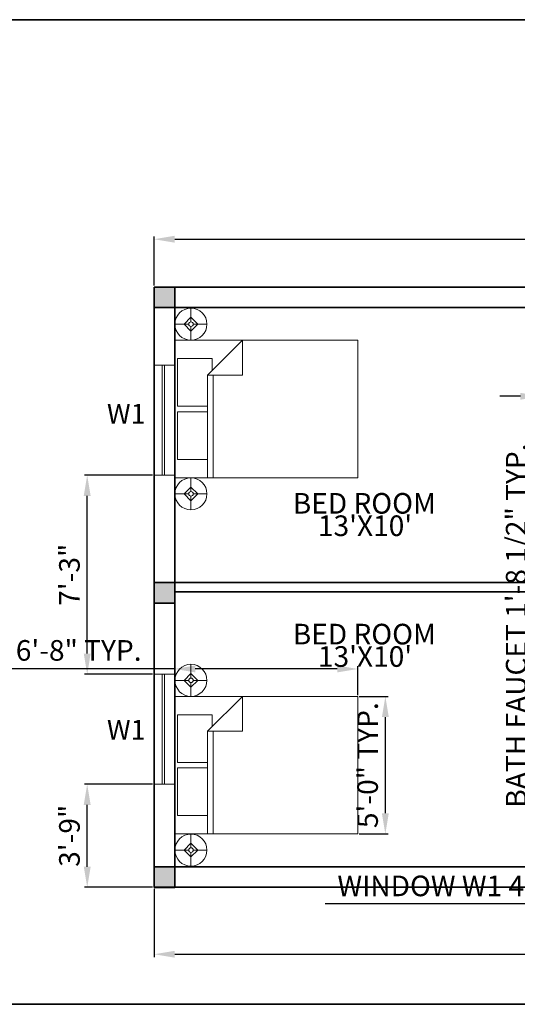
# Model space of a CAD drawing. Units: inches. Extents: x -281 to 2337, y 1647 to 2113.
# Tile 4 of 6: x 1688 to 1906, y 1674 to 2103. Entities that reach past the tile are written whole.
import ezdxf

# ---------------------------------------------------------------- set-up
doc = ezdxf.new("R2010")
doc.units = ezdxf.units.IN
for name, color, linetype, lineweight in [('A-ANNO-DIMS', 242, 'Continuous', 18), ('A-ANNO-IDEN', 11, 'Continuous', 18), ('A-ANNO-TTLB', 7, 'Continuous', 35), ('A-AREA-IDEN', 7, 'Continuous', 18), ('A-COLS', 1, 'Continuous', 35), ('A-FURN', 8, 'Continuous', 18), ('A-GLAZ', 3, 'Continuous', 18), ('A-WALL', 7, 'Continuous', 35)]:
    doc.layers.add(name, color=color, linetype=linetype, lineweight=lineweight)
doc.styles.get("Standard").update_dxf_attribs({"font": 'arial.ttf'})
doc.dimstyles.new('ISO-25', dxfattribs={"dimtxt": 9, "dimasz": 9, "dimexe": 1.25, "dimexo": 0.625, "dimgap": 2, "dimtad": 1, "dimdec": 1, "dimlunit": 4, "dimtxsty": 'Standard', "dimcen": 2.5, "dimadec": 0, "dimazin": 0, "dimtfac": 1, "dimtdec": 1, "dimtmove": 0, "dimatfit": 3, "dimfxl": 1, "dimarcsym": 0})

# ---------------------------------------------------------------- blocks, each defined once
blk = doc.blocks.new('Bed - Queen')
for p, q in [((0, -80.00003), (0, 0)), ((0, 0), (59.99999, 0)), ((59.99999, 0), (59.99999, -80.00003)), ((7.99999, -1.2), (28.79998, -1.2)), ((7.99999, -14.4), (7.99999, -1.2)), ((28.79998, -1.2), (28.79998, -14.4)), ((31.19999, -1.2), (51.99999, -1.2)), ((31.19999, -14.4), (31.19999, -1.2)), ((51.99999, -1.2), (51.99999, -16.4)), ((0, -14.4), (44.8, -14.4)), ((44.8, -16.8), (0, -16.8)), ((59.99999, -29.6), (44.8, -14.4)), ((44.8, -14.4), (44.8, -29.6)), ((51.99999, -16.4), (46.79936, -16.4)), ((44.8, -29.6), (59.99999, -29.6)), ((59.99999, -80.00003), (0, -80.00003))]:
    blk.add_line(p, q)
blk = doc.blocks.new('Lamp - Table')
for p, q in [((0, 7), (0, 1)), ((-1, 0), (-7, 0)), ((0, 3), (-3, 0)), ((-3, 0), (0, -3)), ((3, 0), (0, 3)), ((0, -3), (3, 0)), ((1, 0), (7, 0)), ((0, -1), (0, -7))]:
    blk.add_line(p, q)
for radius in [7, 1]:
    blk.add_circle((0, 0), radius)
blk = doc.blocks.new('*D10')
at = {"layer": 'A-ANNO-DIMS', "color": 0, "lineweight": -2, "transparency": 16777216}
for p, q in [((1746.88, 1987.41), (1746.88, 2008.91)), ((1755.88, 2007.66), (2231.88, 2007.66)), ((2240.88, 1987.41), (2240.88, 2008.91))]:
    blk.add_line(p, q, dxfattribs=at)
at = {"layer": 'A-ANNO-DIMS', "color": 0, "transparency": 16777216}
for points in [[(1755.88, 2009.16), (1755.88, 2006.16), (1746.88, 2007.66)], [(2231.88, 2009.16), (2231.88, 2006.16), (2240.88, 2007.66)]]:
    blk.add_solid(points, dxfattribs=at)
at = {"layer": 'Defpoints', "color": 0, "transparency": 16777216}
for p in [(2240.88, 2007.66), (1746.88, 1986.79), (2240.88, 1986.79)]:
    blk.add_point(p, dxfattribs=at)
at = {"layer": 'A-ANNO-DIMS', "color": 0, "transparency": 16777216, "insert": (1993.88, 2014.18), "char_height": 9, "attachment_point": 5}
blk.add_mtext('41\'-2"', dxfattribs=at)
blk = doc.blocks.new('COL-9x9')
h = blk.add_hatch(color=256)
h.dxf.hatch_style = 1
h.paths.add_polyline_path([(9, 9), (0, 9), (0, 0), (9, 0)])
for p, q in [((0, 9), (9, 9)), ((0, 0), (0, 9)), ((9, 9), (9, 0)), ((9, 0), (0, 0))]:
    blk.add_line(p, q)
blk = doc.blocks.new('WIN-W1-48')
for p, q in [((0, 48), (9, 48)), ((3.5, 0), (3.5, 48)), ((4.5, 0), (4.5, 48)), ((0, 0), (9, 0))]:
    blk.add_line(p, q)
blk = doc.blocks.new('*D19')
at = {"layer": 'A-ANNO-DIMS', "color": 0, "lineweight": -2, "transparency": 16777216}
for p, q in [((1970.88, 1724.16), (1970.88, 1716.34)), ((2018.88, 1724.16), (2018.88, 1716.34)), ((1970.88, 1717.59), (1821.64, 1717.59)), ((2009.88, 1717.59), (1979.88, 1717.59))]:
    blk.add_line(p, q, dxfattribs=at)
at = {"layer": 'A-ANNO-DIMS', "color": 0, "transparency": 16777216}
for points in [[(1979.88, 1719.09), (1979.88, 1716.09), (1970.88, 1717.59)], [(2009.88, 1719.09), (2009.88, 1716.09), (2018.88, 1717.59)]]:
    blk.add_solid(points, dxfattribs=at)
at = {"layer": 'Defpoints', "color": 0, "transparency": 16777216}
for p in [(1970.88, 1724.79), (2018.88, 1724.79), (1970.88, 1717.59)]:
    blk.add_point(p, dxfattribs=at)
at = {"layer": 'A-ANNO-DIMS', "color": 0, "transparency": 16777216, "insert": (1891.76, 1724.24), "char_height": 9, "attachment_point": 5}
blk.add_mtext('WINDOW W1 4\'-0" TYP.', dxfattribs=at)
blk = doc.blocks.new('*D25')
at = {"layer": 'A-ANNO-DIMS', "color": 0, "lineweight": -2, "transparency": 16777216}
for p, q in [((1755.88, 1820.1), (1610.49, 1820.1)), ((1755.88, 1808.73), (1755.88, 1821.35)), ((1826.88, 1820.1), (1764.88, 1820.1)), ((1835.88, 1808.73), (1835.88, 1821.35))]:
    blk.add_line(p, q, dxfattribs=at)
at = {"layer": 'A-ANNO-DIMS', "color": 0, "transparency": 16777216}
for points in [[(1764.88, 1821.6), (1764.88, 1818.6), (1755.88, 1820.1)], [(1826.88, 1821.6), (1826.88, 1818.6), (1835.88, 1820.1)]]:
    blk.add_solid(points, dxfattribs=at)
at = {"layer": 'Defpoints', "color": 0, "transparency": 16777216}
for p in [(1755.88, 1820.1), (1755.88, 1808.1), (1835.88, 1808.1)]:
    blk.add_point(p, dxfattribs=at)
at = {"layer": 'A-ANNO-DIMS', "color": 0, "transparency": 16777216, "insert": (1678.68, 1827.03), "char_height": 9, "attachment_point": 5}
blk.add_mtext('QUEEN BED 6\'-8" TYP.', dxfattribs=at)
blk = doc.blocks.new('*D26')
at = {"layer": 'A-ANNO-DIMS', "color": 0, "lineweight": -2, "transparency": 16777216}
for p, q in [((1836.51, 1808.1), (1849.13, 1808.1)), ((1847.88, 1757.1), (1847.88, 1799.1)), ((1836.51, 1748.1), (1849.13, 1748.1))]:
    blk.add_line(p, q, dxfattribs=at)
at = {"layer": 'A-ANNO-DIMS', "color": 0, "transparency": 16777216}
for points in [[(1846.38, 1799.1), (1849.38, 1799.1), (1847.88, 1808.1)], [(1846.38, 1757.1), (1849.38, 1757.1), (1847.88, 1748.1)]]:
    blk.add_solid(points, dxfattribs=at)
at = {"layer": 'Defpoints', "color": 0, "transparency": 16777216}
for p in [(1835.88, 1808.1), (1847.88, 1808.1), (1835.88, 1748.1)]:
    blk.add_point(p, dxfattribs=at)
at = {"layer": 'A-ANNO-DIMS', "color": 0, "transparency": 16777216, "insert": (1841.29, 1778.1), "char_height": 9, "attachment_point": 5, "rotation": 90}
blk.add_mtext('5\'-0" TYP.', dxfattribs=at)
blk = doc.blocks.new('*D39')
at = {"layer": 'A-ANNO-DIMS', "color": 0, "lineweight": -2, "transparency": 16777216}
for p, q in [((1912.84, 1971.43), (1912.84, 1980.43)), ((1915.26, 1962.43), (1911.59, 1962.43)), ((1912.84, 1962.43), (1912.84, 1942.15)), ((1915.26, 1942.15), (1911.59, 1942.15)), ((1912.84, 1933.15), (1912.84, 1753.91))]:
    blk.add_line(p, q, dxfattribs=at)
at = {"layer": 'A-ANNO-DIMS', "color": 0, "transparency": 16777216}
for points in [[(1911.34, 1971.43), (1914.34, 1971.43), (1912.84, 1962.43)], [(1911.34, 1933.15), (1914.34, 1933.15), (1912.84, 1942.15)]]:
    blk.add_solid(points, dxfattribs=at)
at = {"layer": 'Defpoints', "color": 0, "transparency": 16777216}
for p in [(1915.88, 1962.43), (1912.84, 1942.15), (1915.88, 1942.15)]:
    blk.add_point(p, dxfattribs=at)
at = {"layer": 'A-ANNO-DIMS', "color": 0, "transparency": 16777216, "insert": (1906.19, 1839.03), "char_height": 9, "attachment_point": 5, "rotation": 90}
blk.add_mtext('BATH FAUCET 1\'-8 1/2" TYP.', dxfattribs=at)
blk = doc.blocks.new('*D40')
at = {"layer": 'A-ANNO-DIMS', "color": 0, "lineweight": -2, "transparency": 16777216}
for p, q in [((1906.88, 1939.11), (1897.88, 1939.11)), ((1915.88, 1941.53), (1915.88, 1937.86)), ((1915.88, 1939.11), (1925.01, 1939.11)), ((1925.01, 1941.53), (1925.01, 1937.86)), ((1934.01, 1939.11), (2001.87, 1939.11))]:
    blk.add_line(p, q, dxfattribs=at)
at = {"layer": 'A-ANNO-DIMS', "color": 0, "transparency": 16777216}
for points in [[(1906.88, 1940.61), (1906.88, 1937.61), (1915.88, 1939.11)], [(1934.01, 1940.61), (1934.01, 1937.61), (1925.01, 1939.11)]]:
    blk.add_solid(points, dxfattribs=at)
at = {"layer": 'Defpoints', "color": 0, "transparency": 16777216}
for p in [(1915.88, 1942.15), (1925.01, 1942.15), (1925.01, 1939.11)]:
    blk.add_point(p, dxfattribs=at)
at = {"layer": 'A-ANNO-DIMS', "color": 0, "transparency": 16777216, "insert": (1972.44, 1945.7), "char_height": 9, "attachment_point": 5}
blk.add_mtext('0\'-9" TYP.', dxfattribs=at)
blk = doc.blocks.new('*D41')
at = {"layer": 'A-ANNO-DIMS', "color": 0, "lineweight": -2, "transparency": 16777216}
for p, q in [((1746.88, 1724.16), (1746.88, 1694.33)), ((2267.88, 1724.16), (2267.88, 1694.33)), ((1755.88, 1695.58), (2258.88, 1695.58))]:
    blk.add_line(p, q, dxfattribs=at)
at = {"layer": 'A-ANNO-DIMS', "color": 0, "transparency": 16777216}
for points in [[(1755.88, 1697.08), (1755.88, 1694.08), (1746.88, 1695.58)], [(2258.88, 1697.08), (2258.88, 1694.08), (2267.88, 1695.58)]]:
    blk.add_solid(points, dxfattribs=at)
at = {"layer": 'Defpoints', "color": 0, "transparency": 16777216}
for p in [(1746.88, 1724.79), (2267.88, 1724.79), (2267.88, 1695.58)]:
    blk.add_point(p, dxfattribs=at)
at = {"layer": 'A-ANNO-DIMS', "color": 0, "transparency": 16777216, "insert": (2007.38, 1702.18), "char_height": 9, "attachment_point": 5}
blk.add_mtext('43\'-5"', dxfattribs=at)
blk = doc.blocks.new('*D45')
at = {"layer": 'A-ANNO-DIMS', "color": 0, "lineweight": -2, "transparency": 16777216}
for p, q in [((1746.26, 1769.79), (1716.43, 1769.79)), ((1717.68, 1733.79), (1717.68, 1760.79)), ((1746.26, 1724.79), (1716.43, 1724.79))]:
    blk.add_line(p, q, dxfattribs=at)
at = {"layer": 'A-ANNO-DIMS', "color": 0, "transparency": 16777216}
for points in [[(1716.18, 1760.79), (1719.18, 1760.79), (1717.68, 1769.79)], [(1716.18, 1733.79), (1719.18, 1733.79), (1717.68, 1724.79)]]:
    blk.add_solid(points, dxfattribs=at)
at = {"layer": 'Defpoints', "color": 0, "transparency": 16777216}
for p in [(1717.68, 1769.79), (1746.88, 1769.79), (1746.88, 1724.79)]:
    blk.add_point(p, dxfattribs=at)
at = {"layer": 'A-ANNO-DIMS', "color": 0, "transparency": 16777216, "insert": (1711.08, 1747.29), "char_height": 9, "attachment_point": 5, "rotation": 90}
blk.add_mtext('3\'-9"', dxfattribs=at)
blk = doc.blocks.new('*D46')
at = {"layer": 'A-ANNO-DIMS', "color": 0, "lineweight": -2, "transparency": 16777216}
for p, q in [((1746.26, 1904.66), (1716.43, 1904.66)), ((1717.68, 1826.79), (1717.68, 1895.66)), ((1746.26, 1817.79), (1716.43, 1817.79))]:
    blk.add_line(p, q, dxfattribs=at)
at = {"layer": 'A-ANNO-DIMS', "color": 0, "transparency": 16777216}
for points in [[(1716.18, 1895.66), (1719.18, 1895.66), (1717.68, 1904.66)], [(1716.18, 1826.79), (1719.18, 1826.79), (1717.68, 1817.79)]]:
    blk.add_solid(points, dxfattribs=at)
at = {"layer": 'Defpoints', "color": 0, "transparency": 16777216}
for p in [(1717.68, 1904.66), (1746.88, 1904.66), (1746.88, 1817.79)]:
    blk.add_point(p, dxfattribs=at)
at = {"layer": 'A-ANNO-DIMS', "color": 0, "transparency": 16777216, "insert": (1711.08, 1861.22), "char_height": 9, "attachment_point": 5, "rotation": 90}
blk.add_mtext('7\'-3"', dxfattribs=at)

msp = doc.modelspace()

# ---------------------------------------------------------------- linework, layer by layer
at = {"layer": 'A-ANNO-TTLB'}
msp.add_lwpolyline([(1037.79, 2103.48), (2323.1, 2103.48), (2323.1, 1673.73), (1037.79, 1673.73)], close=True, dxfattribs=at)
at = {"layer": 'A-WALL'}
for p, q in [((1746.88, 1986.79), (2240.88, 1986.79)), ((1746.88, 1724.79), (1746.88, 1986.79)), ((1755.88, 1977.79), (1911.88, 1977.79)), ((1755.88, 1857.79), (1755.88, 1977.79)), ((1915.88, 1857.79), (1746.88, 1857.79)), ((1755.88, 1733.79), (1755.88, 1853.79)), ((1915.88, 1853.79), (1755.88, 1853.79)), ((1911.88, 1733.79), (1755.88, 1733.79)), ((2267.88, 1724.79), (1746.88, 1724.79))]:
    msp.add_line(p, q, dxfattribs=at)

# ---------------------------------------------------------------- block references
at = {"layer": 'A-COLS', "rotation": 180}
for p in [(1755.88, 1986.79), (1755.88, 1857.79), (1755.88, 1733.78)]:
    msp.add_blockref('COL-9x9', p, dxfattribs=at)
at = {"layer": 'A-FURN'}
for name, p, rotation in [('Lamp - Table', (1762.99, 1970.58), 180), ('Bed - Queen', (1755.88, 1903.56), 89.99999999999999), ('Lamp - Table', (1762.99, 1896.51), 180), ('Lamp - Table', (1762.99, 1815.13), 180), ('Bed - Queen', (1755.88, 1748.1), 89.99999999999999), ('Lamp - Table', (1762.99, 1741.05), 180)]:
    msp.add_blockref(name, p, dxfattribs=dict(at, rotation=rotation))
at = {"layer": 'A-GLAZ'}
for p in [(1746.88, 1904.66), (1746.88, 1769.79)]:
    msp.add_blockref('WIN-W1-48', p, dxfattribs=at)

# ---------------------------------------------------------------- texts
at = {"layer": 'A-ANNO-IDEN'}
for p in [(1726.3, 1927.18), (1726.3, 1789.25)]:
    msp.add_text('W1', height=8.623, dxfattribs=at).set_placement(p)
at = {"layer": 'A-AREA-IDEN'}
for s, p in [('BED ROOM ', (1807.45, 1887.89)), ("    13'X10'", (1807.45, 1878.11)), ('BED ROOM ', (1807.45, 1830.81)), ("    13'X10'", (1807.45, 1821.03))]:
    msp.add_text(s, height=9, dxfattribs=at).set_placement(p)

# ---------------------------------------------------------------- dimensions: what is measured, and where the dimension line sits
at = {"layer": 'A-ANNO-DIMS'}
for base, p1, p2, override, picture, middle in [((2240.88, 2007.66), (1746.88, 1986.79), (2240.88, 1986.79), {"dimclrd": 0, "dimclre": 0, "dimclrt": 0}, '*D10', (1993.88, 2014.18)), ((2267.88, 1695.58), (1746.88, 1724.79), (2267.88, 1724.79), {"dimdec": 1, "dimlfac": 1, "dimrnd": 0, "dimzin": 1, "dimdsep": 46, "dimlunit": 4, "dimfrac": 2}, '*D41', (2007.38, 1702.18))]:
    dim = msp.add_linear_dim(base=base, p1=p1, p2=p2, dimstyle='ISO-25', override=override, dxfattribs=at)
    dim.commit()
    dim.dimension.update_dxf_attribs({"geometry": picture, "text_midpoint": middle})
for base, p1, p2, angle, text, picture, middle in [((1912.84, 1942.15), (1915.88, 1962.43), (1915.88, 1942.15), 270, 'BATH FAUCET <> TYP.', '*D39', (1906.19, 1839.03)), ((1755.88, 1820.1), (1835.88, 1808.1), (1755.88, 1808.1), 180, 'QUEEN BED <> TYP.', '*D25', (1678.68, 1827.03)), ((1847.88, 1808.1), (1835.88, 1748.1), (1835.88, 1808.1), 90, '<> TYP.', '*D26', (1841.29, 1778.1)), ((1970.88, 1717.59), (2018.88, 1724.79), (1970.88, 1724.79), 180, 'WINDOW W1 <> TYP.', '*D19', (1891.76, 1724.24))]:
    dim = msp.add_linear_dim(base=base, p1=p1, p2=p2, angle=angle, text=text, dimstyle='ISO-25', override={"dimdec": 1, "dimlfac": 1, "dimrnd": 0, "dimzin": 1, "dimdsep": 46, "dimlunit": 4, "dimfrac": 2}, dxfattribs=at)
    dim.commit()
    dim.dimension.update_dxf_attribs({"geometry": picture, "text_midpoint": middle})
dim = msp.add_linear_dim(base=(1925.01, 1939.11), p1=(1915.88, 1942.15), p2=(1925.01, 1942.15), text='<> TYP.', dimstyle='ISO-25', override={"dimdec": 1, "dimlfac": 1, "dimrnd": 0, "dimzin": 1, "dimdsep": 46, "dimlunit": 4, "dimfrac": 2}, dxfattribs=at)
dim.commit()
dim.dimension.update_dxf_attribs({"geometry": '*D40', "text_midpoint": (1972.44, 1945.7)})
for base, p1, p2, picture, middle in [((1717.68, 1904.66), (1746.88, 1817.79), (1746.88, 1904.66), '*D46', (1711.08, 1861.22)), ((1717.68, 1769.79), (1746.88, 1724.79), (1746.88, 1769.79), '*D45', (1711.08, 1747.29))]:
    dim = msp.add_linear_dim(base=base, p1=p1, p2=p2, angle=90, dimstyle='ISO-25', override={"dimdec": 1, "dimlfac": 1, "dimrnd": 0, "dimzin": 1, "dimdsep": 46, "dimlunit": 4, "dimfrac": 2}, dxfattribs=at)
    dim.commit()
    dim.dimension.update_dxf_attribs({"geometry": picture, "text_midpoint": middle})

doc.saveas('drawing.dxf')
